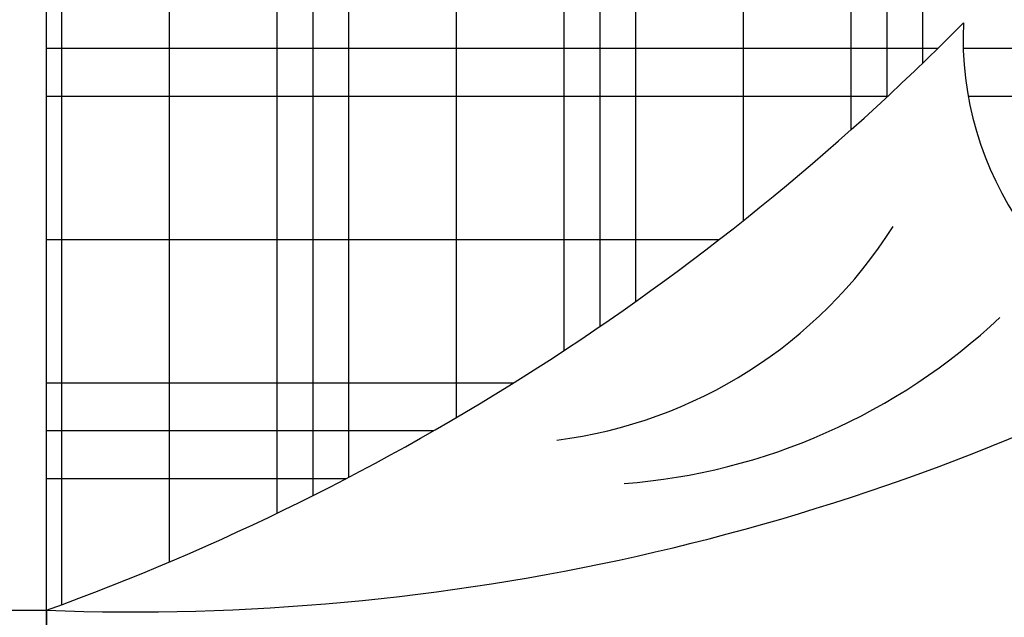
# Model space of a CAD drawing. Units: millimetres. Extents: x 2817 to 5038, y 1110 to 3565.
# Tile 5 of 21: x 2870 to 2917, y 1294 to 1323. Entities that reach past the tile are written whole.
import ezdxf

# ---------------------------------------------------------------- set-up
doc = ezdxf.new("R2010")
doc.units = ezdxf.units.MM
doc.layers.add('BLOCK', color=6, linetype='Continuous')
doc.layers.add('FURNITURE', color=219, linetype='Continuous', lineweight=18)

# ---------------------------------------------------------------- blocks, each defined once
blk = doc.blocks.new('*X7')
at = {"color": 0}
for p, q in [((276.598, 451.25), (280.51, 451.25)), ((275.455, 450.625), (280.51, 450.625)), ((274.411, 450), (280.51, 450)), ((271.723, 448.125), (280.51, 448.125)), ((265.51, 446.25), (268.465, 446.25)), ((269.519, 446.25), (280.51, 446.25)), ((265.51, 445.625), (268.531, 445.625)), ((268.866, 445.625), (280.51, 445.625))]:
    blk.add_line(p, q, dxfattribs=at)
blk = doc.blocks.new('*X8')
at = {"color": 0}
for p, q in [((280.312, 439.886), (280.312, 452.896)), ((278.906, 439.482), (278.906, 452.338)), ((277.5, 439.482), (277.5, 451.702)), ((277.031, 439.482), (277.031, 451.471)), ((276.562, 439.482), (276.562, 451.231)), ((275.156, 439.482), (275.156, 450.451)), ((273.75, 439.482), (273.75, 449.576)), ((273.281, 439.482), (273.281, 449.261)), ((272.812, 439.482), (272.812, 448.934)), ((271.406, 439.482), (271.406, 447.876)), ((270, 439.482), (270, 446.689)), ((269.531, 439.482), (269.531, 446.262)), ((269.062, 439.482), (269.062, 445.817))]:
    blk.add_line(p, q, dxfattribs=at)
blk = doc.blocks.new('A$C52E67D0D')
at = {"layer": 'BLOCK'}
blk.add_lwpolyline([(1901, 0), (601, 0, -0.414214), (501, 100), (501, 1700, -0.414214), (601, 1800), (1901, 1800, -0.414214), (2001, 1700), (2001, 100, -0.414214)], format="xyb", close=True, dxfattribs=at)
blk.add_lwpolyline([(2001, 1348.6), (2001, 1799.6), (2502, 1799.6), (2502, 1348.6)], close=True, dxfattribs=at)
for centre, radius, start, end in [((1888.6, -1664.5), 3015.3, 87.8642, 117.4001), ((3101, -1685.8), 3227.7, 109.926, 135.3977), ((1308.8, 377.9), 807.6, 94.4436, 133.2788), ((1410.8, 520.2), 610.8, 97.2157, 147.6656), ((371.4, 600.4), 432, 357.3792, 72.5379)]:
    blk.add_arc(centre, radius, start, end, dxfattribs=at)
at = {"layer": 'BLOCK', "xscale": 100, "yscale": 100, "zscale": 100}
for name in ['*X8', '*X7']:
    blk.add_blockref(name, (-26050, -43948.2), dxfattribs=at)

msp = doc.modelspace()

# ---------------------------------------------------------------- block references
at = {"layer": 'FURNITURE', "xscale": 0.0367705835331598, "yscale": 0.0367705835331598, "zscale": 0.0367705835331598, "rotation": 180}
msp.add_blockref('A$C52E67D0D', (2944.6948, 1344.1495), dxfattribs=at)

doc.saveas('drawing.dxf')
